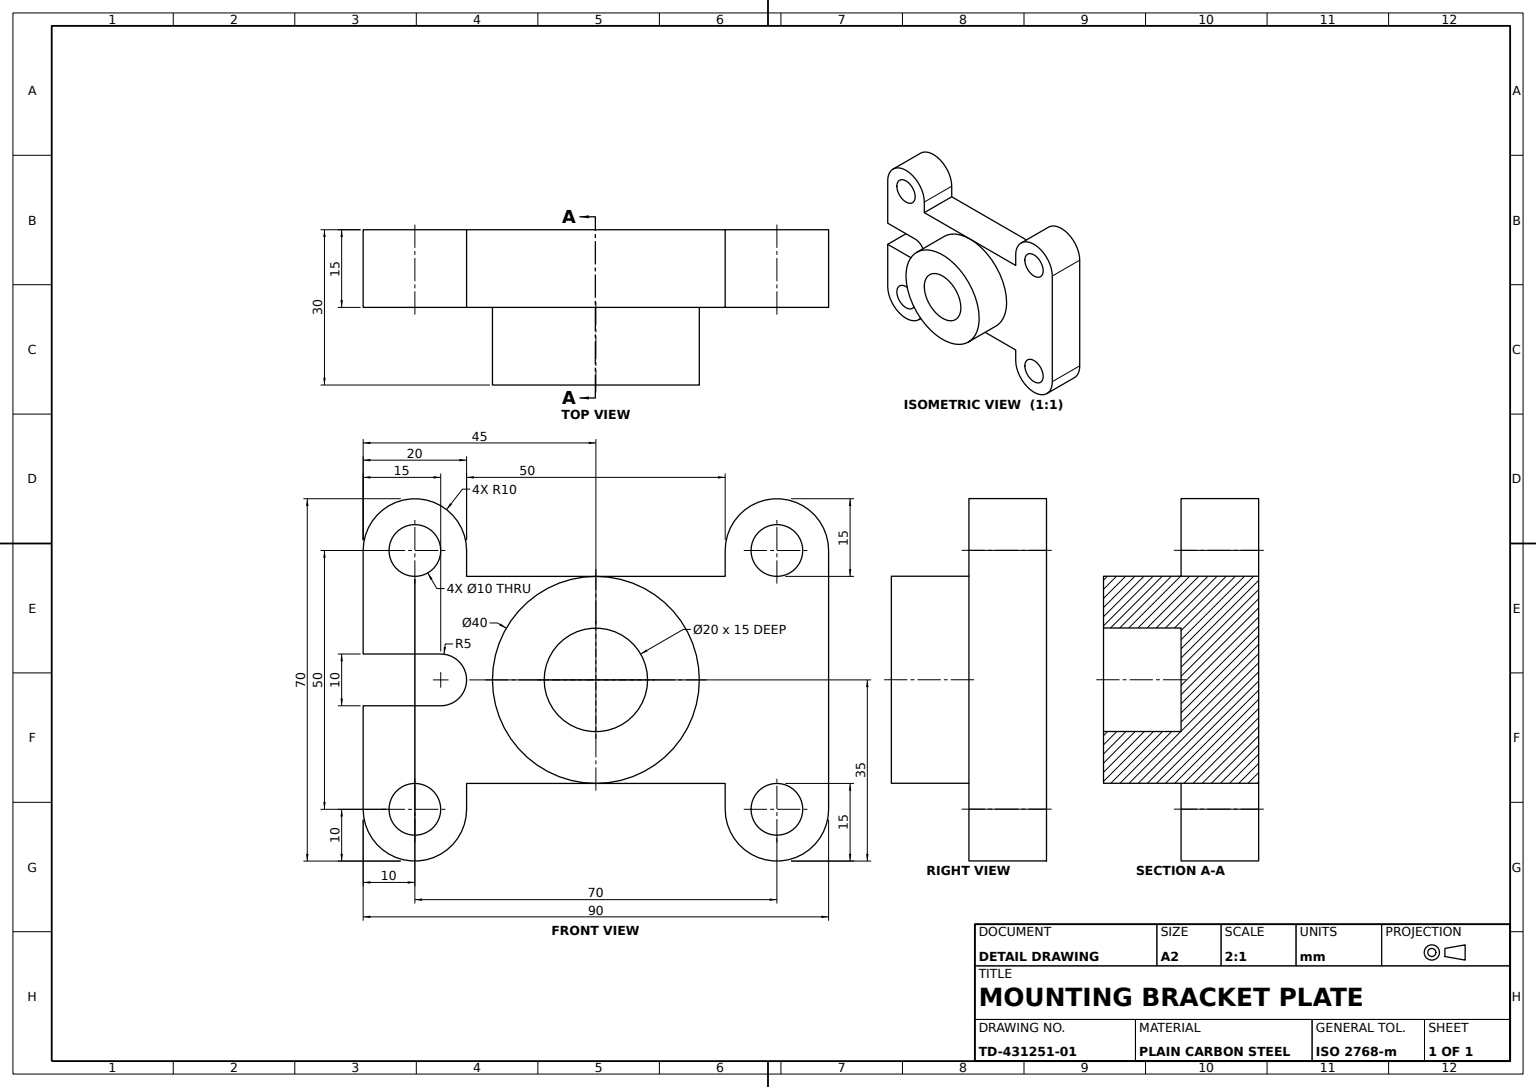
SolidWorks part; units mm, degrees
material "Plain Carbon Steel"
ref_plane "Front Plane" through (0, 0, 0) normal (0, 0, 1) x (1, 0, 0)
ref_plane "Top Plane" through (0, 0, 0) normal (0, 1, 0) x (1, 0, 0)
ref_plane "Right Plane" through (0, 0, 0) normal (1, 0, 0) x (0, 0, -1)
sketch "Base Plate Sketch" plane through (0, 0, 0) normal (0, 0, 1) x (1, 0, 0)
  line L1 (-10, 50) -> (-10, 0)
  line L2 (10, 0) -> (10, 10)
  line L3 (10, 40) -> (10, 50)
  line L4 (0, 50) -> (10, 50)
  line L5 (80, 50) -> (80, 0)
  line L6 (60, 0) -> (60, 10)
  line L7 (60, 10) -> (10, 10)
  line L8 (60, 50) -> (60, 40)
  line L9 (60, 40) -> (10, 40)
  arc A0 (-10, 0) -> (10, 0) centre (0, 0) ccw
  arc A1 (10, 50) -> (-10, 50) centre (0, 50) ccw
  arc A2 (80, 50) -> (60, 50) centre (70, 50) ccw
  arc A3 (60, 0) -> (80, 0) centre (70, 0) ccw
  dimension "D1" = 20
  dimension "D2" = 20
  dimension "D3" = 20
  dimension "D4" = 20
  dimension "D5" = 70
  dimension "D6" = 50
extrude "Base Plate" add sketch "Base Plate Sketch" along normal blind 15
sketch "End Pad 1 Sketch" plane through (0, 40, 0) normal (0, 1, 0) x (1, 0, 0)
  line L0 (10, 0) -> (60, 0)
  line L1 (60, 0) -> (60, -15)
  line L2 (60, -15) -> (10, -15)
  line L3 (10, -15) -> (10, 0)
extrude "End Pad 1" add sketch "End Pad 1 Sketch" along normal blind 5
sketch "End Pad 2 Sketch" plane through (0, 10, 0) normal (0, -1, 0) x (1, 0, 0)
  line L0 (10, 15) -> (60, 15)
  line L1 (60, 15) -> (60, 0)
  line L2 (60, 0) -> (10, 0)
  line L3 (10, 0) -> (10, 15)
extrude "End Pad 2" add sketch "End Pad 2 Sketch" along normal blind 5
sketch "Hub Sketch" plane through (0, 0, 15) normal (0, 0, 1) x (1, 0, 0)
  line L0 (-10, 50) -> (-10, 0) construction
  line L1 (10, 45) -> (60, 45) construction
  circle A0 centre (35, 25) radius 20
  dimension "D1" = 40
  dimension "D2" = 40
  dimension "D3" = 45
  dimension "D4" = 20
extrude "Hub Ø40" add sketch "Hub Sketch" along normal blind 15
sketch "Bore Sketch" plane through (0, 0, 30) normal (0, 0, 1) x (1, 0, 0)
  circle A0 centre (35, 25) radius 10
  dimension "D1" = 20
  dimension "D2" = 20
extrude "Bore Ø20" cut sketch "Bore Sketch" against normal blind 15
sketch "Mounting Holes Sketch" plane through (0, 0, 15) normal (0, 0, 1) x (1, 0, 0)
  circle A0 centre (70, 50) radius 5
  circle A1 centre (70, 0) radius 5
  circle A2 centre (0, 0) radius 5
  circle A3 centre (0, 50) radius 5
  dimension "D1" = 10
  dimension "D2" = 10
  dimension "D3" = 10
  dimension "D4" = 10
  dimension "D5" = 10
extrude "Mounting Holes 4xØ10" cut sketch "Mounting Holes Sketch" against normal blind 15
sketch "Side Notch Sketch" plane through (0, 0, 15) normal (0, 0, 1) x (1, 0, 0)
  line L0 (-10, 30) -> (-10, 20)
  line L1 (-10, 50) -> (-10, 0) construction
  line L2 (5, 30) -> (-10, 30)
  line L3 (5, 20) -> (-10, 20)
  line L4 (10, 45) -> (10, 50) construction
  line L5 (10, 45) -> (35, 45) construction
  arc A0 (5, 20) -> (5, 30) centre (5, 25) ccw
  dimension "D1" = 10
  dimension "D2" = 5
  dimension "D3" = 5
  dimension "D4" = 20
extrude "Side Notch" cut sketch "Side Notch Sketch" against normal blind 15
